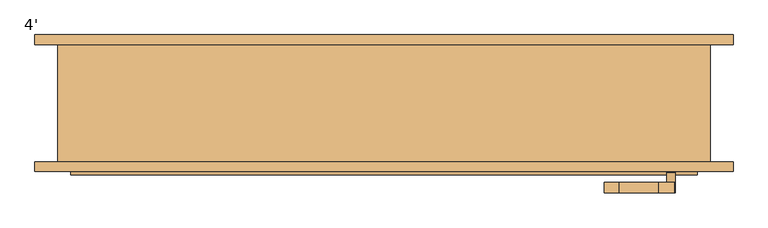
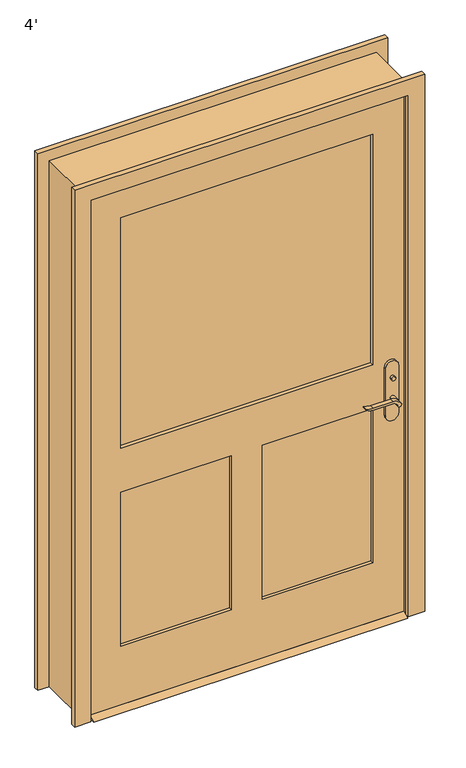
"""IFC4 building model written with IfcOpenShell, lengths in millimetres: door geometry, 4'."""

from ifc_helpers import new_model, si_unit, point, frame, frame_2d, origin, place, context, project, spatial, polyline, circle_curve, trimmed, segment, composite_curve, outline, extrude, faceted_brep, source, transform, mapped, element, save


def door_4_f719ca0b(model_context):
    return source(origin(), model_context, "Body", "SolidModel", [
        extrude(outline(polyline([(-76.2, 12.7), (-50.8, 0.0), (-136.525, 0.0), (-111.125, 12.7), (-76.2, 12.7)])), frame((-609.6, 0.0, 0.0), z_axis=(1.0, 0.0, 0.0), x_axis=(0.0, 1.0, 0.0)), (0.0, 0.0, 1.0), 1219.2),
        extrude(outline(polyline([(563.8, -56.2), (563.8, -66.2), (553.8, -66.2), (553.8, -56.2), (563.8, -56.2)])), frame((0.0, 0.0, 981.9), z_axis=(0.0, 0.0, 1.0), x_axis=(1.0, 0.0, 0.0)), (0.0, 0.0, 1.0), 30.0),
        extrude(outline(composite_curve([segment(trimmed(circle_curve(frame_2d((996.9, 558.8)), 8.0), [point((996.9, 550.8))], [point((996.9, 566.8))], False, "CARTESIAN"), True, "CONTINUOUS"), segment(trimmed(circle_curve(frame_2d((996.9, 558.8)), 8.0), [point((996.9, 566.8))], [point((996.9, 550.8))], False, "CARTESIAN"), True, "CONTINUOUS")], self_intersect=False)), frame((0.0, -131.125, 0.0), z_axis=(0.0, 1.0, 0.0), x_axis=(0.0, 0.0, 1.0)), (0.0, 0.0, 1.0), 10.0),
        extrude(outline(composite_curve([segment(trimmed(circle_curve(frame_2d((897.1555521, 535.1324871)), 37.2832219), [point((919.0523287, 565.3081363))], [point((934.4, 533.4325667))], False, "CARTESIAN"), True, "CONTINUOUS"), segment(polyline([(934.4, 533.4325667), (934.4, 457.1564091)]), True, "CONTINUOUS"), segment(trimmed(circle_curve(frame_2d((1017.6850638, 457.2227909)), 83.2850902), [point((934.4, 457.1564091))], [point((939.4, 428.8))], True, "CARTESIAN"), True, "CONTINUOUS"), segment(polyline([(939.4, 428.8), (936.6135558, 428.8)]), True, "CONTINUOUS"), segment(trimmed(circle_curve(frame_2d((986.6709207, 460.7396612)), 59.3791355), [point((936.6135558, 428.8))], [point((927.4, 457.1564091))], False, "CARTESIAN"), True, "CONTINUOUS"), segment(polyline([(927.4, 457.1564091), (927.4, 533.4138099)]), True, "CONTINUOUS"), segment(trimmed(circle_curve(frame_2d((909.2738613, 533.4138099)), 18.1261387), [point((927.4, 533.4138099))], [point((914.4, 550.8))], True, "CARTESIAN"), True, "CONTINUOUS"), segment(trimmed(circle_curve(frame_2d((914.4, 558.8)), 8.0), [point((914.4, 550.8))], [point((919.0523287, 565.3081363))], False, "CARTESIAN"), True, "CONTINUOUS")], self_intersect=False)), frame((0.0, -36.2, 0.0), z_axis=(0.0, 1.0, 0.0), x_axis=(0.0, 0.0, 1.0)), (0.0, 0.0, 1.0), 20.0),
        extrude(outline(composite_curve([segment(trimmed(circle_curve(frame_2d((914.4, 558.8)), 8.0), [point((914.3999903, 550.8))], [point((919.0523287, 565.3081363))], False, "CARTESIAN"), True, "CONTINUOUS"), segment(trimmed(circle_curve(frame_2d((897.1555521, 535.1324871)), 37.2832219), [point((919.0523287, 565.3081363))], [point((934.4, 533.4325667))], False, "CARTESIAN"), True, "CONTINUOUS"), segment(polyline([(934.4, 533.4325667), (934.4, 457.1564091)]), True, "CONTINUOUS"), segment(trimmed(circle_curve(frame_2d((1017.6850638, 457.2227909)), 83.2850902), [point((934.4, 457.1564091))], [point((939.4, 428.8))], True, "CARTESIAN"), True, "CONTINUOUS"), segment(polyline([(939.4, 428.8), (936.6135558, 428.8)]), True, "CONTINUOUS"), segment(trimmed(circle_curve(frame_2d((986.6709207, 460.7396612)), 59.3791355), [point((936.6135558, 428.8))], [point((927.4, 457.1564091))], False, "CARTESIAN"), True, "CONTINUOUS"), segment(polyline([(927.4, 457.1564091), (927.4, 533.4138122)]), True, "CONTINUOUS"), segment(trimmed(circle_curve(frame_2d((909.2738682, 533.4138122)), 18.1261318), [point((927.4, 533.4138122))], [point((914.3999903, 550.8))], True, "CARTESIAN"), True, "CONTINUOUS")], self_intersect=False)), frame((0.0, -171.125, 0.0), z_axis=(0.0, 1.0, 0.0), x_axis=(0.0, 0.0, 1.0)), (0.0, 0.0, 1.0), 20.0),
        extrude(outline(composite_curve([segment(trimmed(circle_curve(frame_2d((914.4, 558.8)), 8.0), [point((914.4, 550.8))], [point((914.4, 566.8))], False, "CARTESIAN"), True, "CONTINUOUS"), segment(trimmed(circle_curve(frame_2d((914.4, 558.8)), 8.0), [point((914.4, 566.8))], [point((914.4, 550.8))], False, "CARTESIAN"), True, "CONTINUOUS")], self_intersect=False)), frame((0.0, -66.2, 0.0), z_axis=(0.0, 1.0, 0.0), x_axis=(0.0, 0.0, 1.0)), (0.0, 0.0, 1.0), 30.0),
        extrude(outline(composite_curve([segment(trimmed(circle_curve(frame_2d((914.4, 558.8)), 8.0), [point((914.4, 550.8))], [point((914.4, 566.8))], False, "CARTESIAN"), True, "CONTINUOUS"), segment(trimmed(circle_curve(frame_2d((914.4, 558.8)), 8.0), [point((914.4, 566.8))], [point((914.4, 550.8))], False, "CARTESIAN"), True, "CONTINUOUS")], self_intersect=False)), frame((0.0, -151.125, 0.0), z_axis=(0.0, 1.0, 0.0), x_axis=(0.0, 0.0, 1.0)), (0.0, 0.0, 1.0), 30.0),
        extrude(outline(composite_curve([segment(polyline([(844.4, 583.8), (1039.4, 583.8)]), True, "CONTINUOUS"), segment(trimmed(circle_curve(frame_2d((1039.4, 558.8)), 25.0), [point((1039.4, 583.8))], [point((1039.4, 533.8))], False, "CARTESIAN"), True, "CONTINUOUS"), segment(polyline([(1039.4, 533.8), (844.4, 533.8)]), True, "CONTINUOUS"), segment(trimmed(circle_curve(frame_2d((844.4, 558.8)), 25.0), [point((844.4, 533.8))], [point((844.4, 583.8))], False, "CARTESIAN"), True, "CONTINUOUS")], self_intersect=False)), frame((0.0, -76.2, 0.0), z_axis=(0.0, 1.0, 0.0), x_axis=(0.0, 0.0, 1.0)), (0.0, 0.0, 1.0), 10.0),
        extrude(outline(composite_curve([segment(polyline([(844.4, 583.8), (1039.4, 583.8)]), True, "CONTINUOUS"), segment(trimmed(circle_curve(frame_2d((1039.4, 558.8)), 25.0), [point((1039.4, 583.8))], [point((1039.4, 533.8))], False, "CARTESIAN"), True, "CONTINUOUS"), segment(polyline([(1039.4, 533.8), (844.4, 533.8)]), True, "CONTINUOUS"), segment(trimmed(circle_curve(frame_2d((844.4, 558.8)), 25.0), [point((844.4, 533.8))], [point((844.4, 583.8))], False, "CARTESIAN"), True, "CONTINUOUS")], self_intersect=False)), frame((0.0, -121.125, 0.0), z_axis=(0.0, 1.0, 0.0), x_axis=(0.0, 0.0, 1.0)), (0.0, 0.0, 1.0), 10.0),
        extrude(outline(polyline([(2133.6, -609.6), (12.7, -609.6), (12.7, 609.6), (2133.6, 609.6), (2133.6, -609.6)]), holes=[polyline([(1066.8, -488.95), (2012.95, -488.95), (2012.95, 488.95), (1066.8, 488.95), (1066.8, -488.95)]), polyline([(885.825, -60.325), (254.0, -60.325), (254.0, -488.95), (885.825, -488.95), (885.825, -60.325)]), polyline([(885.825, 488.95), (254.0, 488.95), (254.0, 60.325), (885.825, 60.325), (885.825, 488.95)])]), frame((0.0, -111.125, 0.0), z_axis=(0.0, 1.0, 0.0), x_axis=(0.0, 0.0, 1.0)), (0.0, 0.0, 1.0), 34.925),
        faceted_brep([(635.0, -111.125, 0.0), (609.6, -111.125, 0.0), (609.6, -76.2, 0.0), (596.9, -76.2, 0.0), (596.9, -41.275, 0.0), (609.6, -41.275, 0.0), (609.6, 117.475, 0.0), (635.0, 117.475, 0.0), (635.0, 117.475, 2159.0), (635.0, -111.125, 2159.0), (609.6, 117.475, 2133.6), (-609.6, 117.475, 2133.6), (-609.6, 117.475, 0.0), (-635.0, 117.475, 0.0), (-635.0, 117.475, 2159.0), (609.6, -41.275, 2133.6), (596.9, -41.275, 2120.9), (-596.9, -41.275, 2120.9), (-596.9, -41.275, 0.0), (-609.6, -41.275, 0.0), (-609.6, -41.275, 2133.6), (596.9, -76.2, 2120.9), (609.6, -76.2, 2133.6), (-609.6, -76.2, 2133.6), (-609.6, -76.2, 0.0), (-596.9, -76.2, 0.0), (-596.9, -76.2, 2120.9), (609.6, -111.125, 2133.6), (-635.0, -111.125, 2159.0), (-635.0, -111.125, 0.0), (-609.6, -111.125, 0.0), (-609.6, -111.125, 2133.6)], [[[0, 1, 2, 3, 4, 5, 6, 7]], [[7, 8, 9, 0]], [[6, 10, 11, 12, 13, 14, 8, 7]], [[5, 15, 10, 6]], [[4, 16, 17, 18, 19, 20, 15, 5]], [[3, 21, 16, 4]], [[2, 22, 23, 24, 25, 26, 21, 3]], [[1, 27, 22, 2]], [[0, 9, 28, 29, 30, 31, 27, 1]], [[8, 14, 28, 9]], [[15, 20, 11, 10]], [[21, 26, 17, 16]], [[27, 31, 23, 22]], [[29, 13, 12, 19, 18, 25, 24, 30]], [[14, 13, 29, 28]], [[20, 19, 12, 11]], [[26, 25, 18, 17]], [[31, 30, 24, 23]]]),
        extrude(outline(polyline([(-60.325, -87.8416667), (-60.325, -99.4833333), (-488.95, -99.4833333), (-488.95, -87.8416667), (-60.325, -87.8416667)])), frame((0.0, 0.0, 254.0), z_axis=(0.0, 0.0, 1.0), x_axis=(1.0, 0.0, 0.0)), (0.0, 0.0, 1.0), 631.825),
        extrude(outline(polyline([(488.95, -87.8416667), (488.95, -99.4833333), (60.325, -99.4833333), (60.325, -87.8416667), (488.95, -87.8416667)])), frame((0.0, 0.0, 254.0), z_axis=(0.0, 0.0, 1.0), x_axis=(1.0, 0.0, 0.0)), (0.0, 0.0, 1.0), 631.825),
        extrude(outline(polyline([(488.95, -90.17), (488.95, -97.155), (-488.95, -97.155), (-488.95, -90.17), (488.95, -90.17)])), frame((0.0, 0.0, 1066.8), z_axis=(0.0, 0.0, 1.0), x_axis=(1.0, 0.0, 0.0)), (0.0, 0.0, 1.0), 946.15),
        extrude(outline(polyline([(0.0, -615.95), (2139.95, -615.95), (2139.95, 615.95), (0.0, 615.95), (0.0, 679.45), (2203.45, 679.45), (2203.45, -679.45), (0.0, -679.45), (0.0, -615.95)])), frame((0.0, 117.475, 0.0), z_axis=(0.0, 1.0, 0.0), x_axis=(0.0, 0.0, 1.0)), (0.0, 0.0, 1.0), 19.05),
        extrude(outline(polyline([(0.0, -615.95), (2139.95, -615.95), (2139.95, 615.95), (0.0, 615.95), (0.0, 679.45), (2203.45, 679.45), (2203.45, -679.45), (0.0, -679.45), (0.0, -615.95)])), frame((0.0, -130.175, 0.0), z_axis=(0.0, 1.0, 0.0), x_axis=(0.0, 0.0, 1.0)), (0.0, 0.0, 1.0), 19.05),
    ])


if __name__ == "__main__":
    model = new_model("IFC4")
    model_context = context("Model", 3, world=origin())
    ifc_project = project(units=[si_unit("LENGTHUNIT", "METRE", prefix="MILLI")], contexts=[model_context])
    site = spatial("IfcSite", under=ifc_project)
    building = spatial("IfcBuilding", under=site)
    placement = place(None, origin())
    door_4_shape = door_4_f719ca0b(model_context)
    element("IfcDoor", 1, ObjectType="4'", at=placement, inside=building, context=model_context, shape_type="MappedRepresentation", body=[
        mapped(door_4_shape, transform((0.0, 0.0, 0.0), x_axis=(1.0, 0.0, 0.0), y_axis=(0.0, 1.0, 0.0), z_axis=(0.0, 0.0, 1.0))),
    ])
    save(model, "model.ifc")

# Revit data of these elements
# Type "4'"
#   Type Mark = "10"
#   Assembly Code = "B2030100"
#   Analytic Construction = "French door, wood frame with single glass"
#   Top Rail = 0' - 4 3/4"
#   Threshold Offset [instance default] = 0' - 0 1/2"
#   Thickness = 0' - 1 3/8"
#   Thermal Resistance (R) = 1.0696 (h·ft²·°F)/BTU
#   Swing Angle [instance default] = 90.00°
#   Stiles = 0' - 4 3/4"
#   Rough Width = 4' - 2"
#   Rough Height = 7' - 1"
#   Lock Rail = 0' - 7 1/8"
#   Height = 7' - 0"
#   Width = 4' - 0"
#   Heat Transfer Coefficient (U) = 0.9350 BTU/(h·ft²·°F)
#   Door Offset [instance default] = 0' - 0"
#   Bottom Rail = 0' - 9 1/2"
#   Threshold [instance default] = yes
#   Function = 1
#   Exterior Trim [instance default] = yes
#   Trim Material = Cherry
#   Threshold Material = Cherry
#   Panel Material = Cherry
#   Glazing = Glass
#   Frame Material = Cherry
#   Door Handle Material = Aluminum
#   Visual Light Transmittance = 0
#   Solar Heat Gain Coefficient = 0
#   Wall Closure = (empty or 0)
#   Construction Type = (empty or 0)
# Element 1 (IfcDoor, "4'")
#   Materials on its faces: "Cherry", "Aluminum", "Glass"
# Materials
#   "Cherry": class "Wood", colour RGB 226 177 128, transparency 0, Description = "Prunus Serotina", Cost = 0
#   "Glass": class "Glass", colour RGB 0 128 192, transparency 0.75, Description = "Soda Lime Glass", Cost = 0
#   "Aluminum": class "Metal", colour RGB 247 247 247, transparency 0, Description = "Aluminum 6061", Cost = 0
